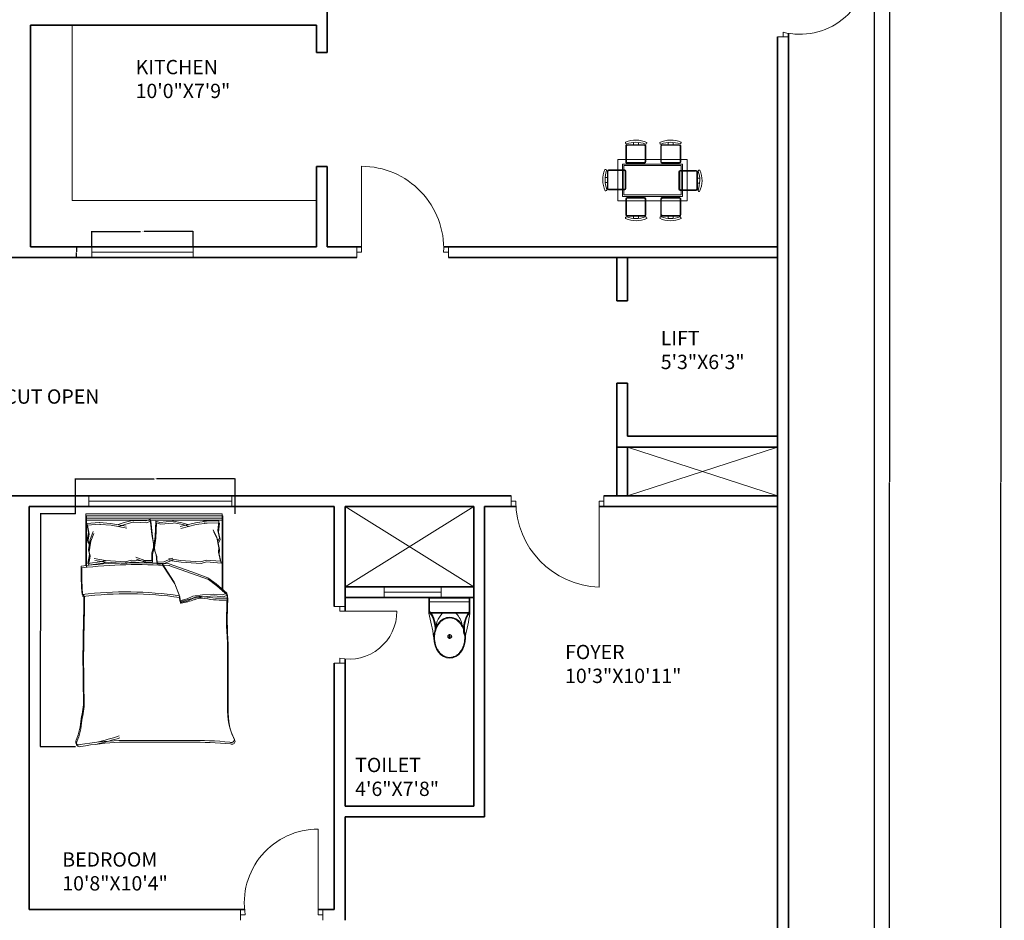
# Model space of a CAD drawing. Units: inches. Extents: x 1520 to 3401, y 1570 to 3432.
# Tile 6 of 15: x 2022 to 2435, y 2061 to 2438. Entities that reach past the tile are written whole.
import ezdxf

# ---------------------------------------------------------------- set-up
doc = ezdxf.new("R2010")
doc.units = ezdxf.units.IN
for name, color, linetype, lineweight in [('A-ANNO-DIMS', 2, 'Continuous', 18), ('A-AREA-IDEN', 7, 'Continuous', 18), ('A-DOOR', 3, 'Continuous', 18), ('A-FLOR-CASE', 8, 'Continuous', 18), ('A-FLOR-EDGE', 7, 'Continuous', 25), ('A-FLOR-EVTR', 7, 'Continuous', 35), ('A-FLOR-FIXT', 9, 'Continuous', 18), ('A-FLOR-OPEN', 8, 'Continuous', 13), ('A-FURN', 8, 'Continuous', 13), ('A-GLAZ', 4, 'Continuous', 18), ('A-WALL', 7, 'Continuous', 35)]:
    doc.layers.add(name, color=color, linetype=linetype, lineweight=lineweight)
doc.styles.get("Standard").update_dxf_attribs({"font": 'arial.ttf'})
doc.dimstyles.get("Standard").update_dxf_attribs({"dimtxt": 0.18, "dimasz": 0.18, "dimexe": 0.18, "dimexo": 0.0625, "dimgap": 0.09, "dimtad": 0, "dimtih": 1, "dimtoh": 1, "dimdec": 4, "dimzin": 0, "dimdsep": 46, "dimtxsty": 'Standard', "dimcen": 0.09, "dimadec": 0, "dimazin": 0, "dimtfac": 1, "dimtdec": 4, "dimtofl": 0, "dimtmove": 0, "dimatfit": 3, "dimfxl": 1, "dimtolj": 1, "dimtzin": 0, "dimarcsym": 0})

# ---------------------------------------------------------------- blocks, each defined once
blk = doc.blocks.new('A$C31115884')
for p, q in [((258, 466), (258, 523)), ((283, 498), (223, 498)), ((0, 200), (0, 0)), ((520, 200), (0, 200)), ((10, 190), (10, 10)), ((510, 190), (10, 190)), ((510, 10), (510, 190)), ((520, 0), (520, 200)), ((510, 54), (0, 54)), ((10, 10), (510, 10)), ((0, 0), (520, 0))]:
    blk.add_line(p, q)
blk.add_circle((256, 496), 23.6)
for centre, radius, start, end in [((2778, -205), 2807, 165.4549, 171.7133), ((3237, 905), 2807, 188.2867, 194.5451), ((-295, 403), 365, 324.2091, 9.3499), ((-295, 403), 375, 324.2091, 9.3499), ((139, 406), 293, 315.8436, 2.6563), ((806, 403), 375, 179.2036, 215.7909), ((806, 403), 365, 170.6501, 215.7909), ((384, 406), 293, 190.2774, 224.1564)]:
    blk.add_arc(centre, radius, start, end)
blk.add_ellipse((256, 510), major_axis=(0, -261), ratio=0.772727)
blk.add_open_spline([(256, 259), (263, 259), (270, 260), (288, 262), (299, 265), (320, 273), (330, 278), (350, 291), (360, 299), (378, 316), (386, 326), (402, 347), (409, 358), (421, 383), (427, 395), (436, 422), (440, 436), (445, 465), (447, 480), (448, 509), (448, 524), (445, 553), (443, 568), (436, 596), (432, 610), (422, 636), (416, 649), (402, 672), (395, 683), (379, 703), (370, 712), (351, 728), (341, 735), (321, 746), (310, 751), (289, 757), (278, 759), (256, 761), (245, 761), (223, 757), (212, 754), (191, 746), (181, 741), (161, 728), (151, 720), (133, 703), (125, 693), (110, 672), (103, 660), (90, 636), (85, 623), (76, 596), (72, 582), (67, 553), (66, 538), (64, 509), (65, 494), (68, 465), (70, 450), (77, 422), (81, 408), (91, 382), (97, 370), (111, 346), (118, 335), (135, 316), (144, 307), (162, 291), (172, 284), (193, 273), (203, 269), (225, 262), (236, 260), (250, 259), (253, 259), (256, 259)], degree=3, knots=[0, 0, 0, 0, 0.110105, 0.110105, 0.285049, 0.285049, 0.459994, 0.459994, 0.634938, 0.634938, 0.809882, 0.809882, 0.984827, 0.984827, 1.159771, 1.159771, 1.334715, 1.334715, 1.50966, 1.50966, 1.684604, 1.684604, 1.859549, 1.859549, 2.034493, 2.034493, 2.209437, 2.209437, 2.384382, 2.384382, 2.559326, 2.559326, 2.73427, 2.73427, 2.909215, 2.909215, 3.084159, 3.084159, 3.259103, 3.259103, 3.434048, 3.434048, 3.608992, 3.608992, 3.783936, 3.783936, 3.958881, 3.958881, 4.133825, 4.133825, 4.30877, 4.30877, 4.483714, 4.483714, 4.658658, 4.658658, 4.833603, 4.833603, 5.008547, 5.008547, 5.183491, 5.183491, 5.358436, 5.358436, 5.53338, 5.53338, 5.708324, 5.708324, 5.883269, 5.883269, 6.058213, 6.058213, 6.233158, 6.233158, 6.283185, 6.283185, 6.283185, 6.283185])
blk = doc.blocks.new('DOOR-SWING-36-16')
for p, q in [((0, 33.75), (0, 38.25)), ((0, 38.25), (0, 36)), ((38.88, 38.25), (38.88, 33.75)), ((0, 36), (2, 36)), ((38.88, 36), (36.88, 36)), ((36.88, 36), (36.88, 0)), ((38.88, 33.75), (38.88, 36)), ((38.88, 36), (38.88, 36))]:
    blk.add_line(p, q)
blk.add_arc((38.02, 36), 36.02, 180, 268.1872)
blk = doc.blocks.new('DOOR-SWING-36-18')
for p, q in [((32.58, 2.25), (32.58, 38.25)), ((0, 4.5), (0, 0)), ((34.58, 4.5), (34.58, 0)), ((0, 0), (0, 2.25)), ((0, 2.25), (2, 2.25)), ((34.58, 2.25), (32.58, 2.25)), ((34.58, 0), (34.58, 2.25))]:
    blk.add_line(p, q)
blk.add_arc((32.58, 7.26), 30.99, 90, 189.3104)
blk = doc.blocks.new('DOOR-SWING-24-19')
for p, q in [((4.5, 23.7), (0, 23.7)), ((0, 23.7), (2.25, 23.7)), ((2.25, 23.7), (2.25, 21.7)), ((2.25, 21.7), (26.25, 21.7)), ((0, 0), (4.5, 0)), ((2.25, 0), (2.25, 2)), ((4.5, 0), (2.25, 0))]:
    blk.add_line(p, q)
blk.add_arc((6.17, 21.7), 20.08, 258.7571, 0)
blk = doc.blocks.new('DOOR-SWING-36-20')
for p, q in [((2, 2.25), (2, 38.25)), ((0, 4.5), (0, 0)), ((38.43, 4.5), (38.43, 0)), ((0, 0), (0, 2.25)), ((0, 2.25), (2, 2.25)), ((38.43, 2.25), (36.43, 2.25)), ((38.43, 0), (38.43, 2.25))]:
    blk.add_line(p, q)
blk.add_arc((2, 3.79), 34.46, 357.4431, 90)
blk = doc.blocks.new('DOOR-SWING-36-23')
for p, q in [((0, 32.12), (4.5, 32.12)), ((4.5, 32.12), (2.25, 32.12)), ((2.25, 32.12), (2.25, 30.12)), ((2.25, 30.12), (38.25, 30.12)), ((4.5, 0), (0, 0)), ((0, 0), (2.25, 0)), ((2.25, 0), (2.25, 2))]:
    blk.add_line(p, q)
blk.add_arc((9.27, 30.12), 28.98, 255.986, 0)
blk = doc.blocks.new('WIN-PLAN-24-01')
for p, q in [((0, 4.5), (0, 0)), ((24, 2.25), (24, 4.5)), ((24, 4.5), (24, 0)), ((0, 0), (0, 2.25)), ((0, 2.25), (24, 2.25))]:
    blk.add_line(p, q)
blk = doc.blocks.new('WIN-PLAN-60-02')
for p, q in [((4.5, 60), (0, 60)), ((0, 60), (2.25, 60)), ((2.25, 60), (2.25, 0)), ((4.5, 0), (0, 0)), ((2.25, 0), (4.5, 0))]:
    blk.add_line(p, q)
blk = doc.blocks.new('WIN-PLAN-42.5-08')
for p, q in [((0, 4.5), (0, 0)), ((42.53, 0), (42.53, 4.5)), ((0, 0), (0, 2.25)), ((0, 2.25), (0, 2.25)), ((0, 2.25), (42.53, 2.25))]:
    blk.add_line(p, q)
blk = doc.blocks.new('BED-DOUBLE')
for p, q in [((4.17, 75.93), (4.17, 97.64)), ((4.17, 97.64), (61.46, 97.64)), ((4.17, 95.8), (61.46, 95.8)), ((4.44, 75.16), (4.44, 96.87)), ((4.44, 96.87), (61.73, 96.87)), ((4.44, 95.03), (61.73, 95.03)), ((29.42, 94.7), (31.15, 95.4)), ((31.15, 95.4), (31.84, 88.98)), ((61.46, 97.64), (61.46, 65.74)), ((61.73, 96.87), (61.73, 64.97)), ((4.67, 93.64), (9.81, 94.03)), ((4.67, 93.66), (5.36, 89.85)), ((4.94, 92.9), (5.64, 89.08)), ((4.95, 92.87), (10.08, 93.27)), ((9.81, 94.03), (9.93, 94.01)), ((9.93, 94.01), (14.52, 93.66)), ((10.08, 93.27), (10.21, 93.24)), ((10.21, 93.24), (14.79, 92.9)), ((14.52, 93.66), (21.1, 92.45)), ((14.79, 92.9), (21.38, 91.68)), ((17.81, 93.14), (20.24, 94.01)), ((18.08, 92.38), (20.51, 93.24)), ((20.24, 94.01), (23.7, 94.88)), ((20.51, 93.24), (23.98, 94.11)), ((23.7, 94.88), (24.09, 94.88)), ((23.98, 94.11), (24.36, 94.11)), ((24.09, 94.88), (29.42, 94.7)), ((24.36, 94.11), (29.69, 93.94)), ((29.69, 93.94), (31.42, 94.63)), ((31.42, 94.63), (32.12, 88.22)), ((33.54, 94.65), (33.25, 88.21)), ((33.81, 93.88), (33.52, 87.44)), ((35.31, 94.07), (33.54, 94.65)), ((35.59, 93.3), (33.81, 93.88)), ((40.62, 94.57), (35.31, 94.07)), ((40.9, 93.81), (35.59, 93.3)), ((41.01, 94.6), (40.62, 94.57)), ((41.28, 93.83), (40.9, 93.81)), ((44.52, 93.95), (41.01, 94.6)), ((44.79, 93.18), (41.28, 93.83)), ((50.25, 93.96), (43.75, 92.34)), ((50.52, 93.19), (44.03, 91.57)), ((47, 93.23), (44.52, 93.95)), ((47.27, 92.47), (44.79, 93.18)), ((54.8, 94.59), (50.25, 93.96)), ((55.08, 93.82), (50.52, 93.19)), ((60.08, 94.57), (53.6, 94.69)), ((53.6, 94.69), (54.8, 94.59)), ((60.35, 93.81), (53.87, 93.92)), ((53.87, 93.92), (55.08, 93.82)), ((59.12, 87.74), (57.7, 90.95)), ((60.08, 94.57), (59.62, 90.72)), ((60.35, 93.81), (59.9, 89.96)), ((5.36, 89.85), (4.84, 86.73)), ((5.64, 89.08), (5.12, 85.96)), ((5.36, 82.57), (6.06, 86.9)), ((6.06, 86.9), (7.27, 90.2)), ((6.33, 86.14), (7.54, 89.43)), ((31.84, 88.98), (32.54, 85.17)), ((32.12, 88.22), (32.81, 84.4)), ((33.25, 88.21), (32.79, 84.36)), ((33.52, 87.44), (33.07, 83.59)), ((59.39, 86.97), (57.97, 90.18)), ((60.08, 83.46), (59.12, 87.74)), ((60.35, 82.69), (59.39, 86.97)), ((59.62, 90.72), (60.34, 87.64)), ((60.34, 87.64), (59.72, 86.39)), ((59.9, 89.96), (60.61, 86.88)), ((60.61, 86.88), (59.99, 85.62)), ((4.84, 86.73), (5.54, 85.52)), ((5.12, 85.96), (5.81, 84.75)), ((5.64, 81.8), (6.33, 86.14)), ((32.54, 83.61), (31.84, 81.36)), ((32.81, 82.84), (32.12, 80.59)), ((32.54, 85.17), (32.54, 83.61)), ((32.79, 84.36), (32.89, 82.8)), ((32.81, 84.4), (32.81, 82.84)), ((32.89, 82.8), (33.72, 80.59)), ((33.07, 83.59), (33.17, 82.03)), ((59.85, 81.53), (60.08, 83.46)), ((60.12, 80.77), (60.35, 82.69)), ((5.02, 76.85), (5.71, 80.66)), ((5.29, 76.08), (5.98, 79.9)), ((5.71, 80.66), (5.36, 82.57)), ((5.98, 79.9), (5.64, 81.8)), ((7.65, 78.9), (12.48, 78.1)), ((28.9, 78.14), (25.13, 79.45)), ((29.17, 77.37), (25.4, 78.68)), ((31.84, 81.36), (31.84, 78.14)), ((32.12, 80.59), (32.12, 77.37)), ((33.17, 82.03), (34, 79.83)), ((33.72, 80.59), (33.93, 77.39)), ((34, 79.83), (34.2, 76.62)), ((36.87, 77.57), (40.55, 79.11)), ((39.04, 78.9), (43.87, 78.1)), ((60.78, 77.77), (59.85, 81.53)), ((61.05, 77), (60.12, 80.77)), ((11.13, 77.72), (5.02, 76.85)), ((11.4, 76.95), (5.29, 76.08)), ((7.92, 78.14), (12.76, 77.34)), ((12.48, 78.1), (11.13, 77.72)), ((12.76, 77.34), (11.4, 76.95)), ((12.48, 78.1), (20.89, 77.59)), ((12.76, 77.34), (21.16, 76.82)), ((20.89, 77.59), (23.24, 78.25)), ((21.16, 76.82), (23.51, 77.49)), ((23.24, 78.25), (29.39, 77.77)), ((23.51, 77.49), (29.67, 77)), ((31.84, 78.14), (28.9, 78.14)), ((32.12, 77.37), (29.17, 77.37)), ((33.93, 77.39), (36.87, 77.57)), ((34.2, 76.62), (37.14, 76.8)), ((36.28, 76.8), (41.3, 69.01)), ((36.55, 76.03), (41.57, 68.25)), ((37.14, 76.8), (40.82, 78.34)), ((48.73, 73.28), (38.73, 76.8)), ((49, 72.52), (39, 76.03)), ((39.31, 78.14), (44.15, 77.34)), ((43.87, 78.1), (52.28, 77.59)), ((44.15, 77.34), (52.55, 76.82)), ((52.28, 77.59), (54.63, 78.25)), ((52.55, 76.82), (54.9, 77.49)), ((54.63, 78.25), (60.78, 77.77)), ((54.9, 77.49), (61.05, 77)), ((55.41, 70.87), (48.73, 73.28)), ((55.69, 70.1), (49, 72.52)), ((58.94, 68.27), (55.41, 70.87)), ((41.3, 69.01), (43.34, 63.63)), ((41.57, 68.25), (43.62, 62.87)), ((59.21, 67.51), (55.69, 70.1)), ((63.38, 64.38), (58.94, 68.27)), ((63.66, 63.61), (59.21, 67.51)), ((43.34, 63.63), (43.71, 61.22)), ((43.62, 62.87), (43.99, 60.45)), ((46.68, 61.96), (49.1, 63.08)), ((46.96, 61.2), (49.37, 62.31)), ((49.1, 63.08), (53.18, 63.63)), ((49.37, 62.31), (53.46, 62.87)), ((53.18, 63.63), (57.82, 64)), ((53.46, 62.87), (58.1, 63.24)), ((57.82, 64), (61.54, 63.63)), ((58.1, 63.24), (61.81, 62.87)), ((61.54, 63.63), (63.38, 64.38)), ((61.81, 62.87), (63.66, 63.61)), ((63.48, 62.28), (63.38, 64.38, 4.64)), ((63.75, 61.52), (63.66, 63.61, 4.64)), ((43.71, 61.22), (46.68, 61.96)), ((43.99, 60.45), (46.96, 61.2)), ((18.06, 2.64), (47.57, 2.64)), ((18.33, 1.87), (47.84, 1.87))]:
    blk.add_line(p, q)
for centre, radius, start, end in [((102.1, 73.55), 99.87, 178.7218, 185.604), ((25.61, -120.62), 197.77, 86.0865, 96.7821), ((102.37, 72.78), 99.87, 178.7218, 185.604), ((25.88, -121.38), 197.77, 86.0865, 96.7821), ((21.29, -89.76), 154.68, 81.7845, 96.9006), ((21.56, -90.53), 154.68, 81.7845, 96.9006), ((-200.58, 60.27), 203.94, 358.4762, 1.0082), ((-200.3, 59.5), 203.94, 358.4762, 1.0082), ((37.35, 95.86), 35.55, 280.6617, 289.8806), ((52.44, 55.6), 7.46, 78.6608, 113.7384), ((52.72, 54.83), 7.46, 78.6608, 113.7384), ((61.53, 105.62), 43.38, 259.8763, 272.5657), ((61.81, 104.85), 43.38, 259.8763, 272.5657), ((218.51, 54.1), 155.25, 176.9791, 183.8365), ((43.92, 61.15), 0.221, 160.2464, 271.1377), ((44.2, 60.38), 0.221, 160.2464, 271.1377), ((37.62, 95.1), 35.55, 280.6617, 289.8806), ((218.79, 53.34), 155.25, 176.9791, 183.8365), ((581.23, 36.96), 578.22, 178.22771, 181.71854), ((581.51, 36.19), 578.22, 178.22771, 181.71854), ((-5405.34, 16.33), 5469.02, 0.00217, 0.28689), ((-5405.07, 15.56), 5469.02, 0.00217, 0.28689), ((-32.25, 20.29), 35.53, 346.0648, 358.9113), ((-31.97, 19.53), 35.53, 346.0648, 358.9113), ((91.3, 15.32), 27.65, 177.4714, 206.4681), ((91.58, 14.55), 27.65, 177.4714, 206.4681), ((-25.97, 13.39), 28.25, 337.9751, 356.652), ((-25.69, 12.62), 28.25, 337.9751, 356.652), ((-20.65, 126.07), 127.63, 283.3832, 287.7053), ((1.3, 2.07), 1.31, 146.1736, 293.4781), ((1.58, 1.3), 1.31, 146.1736, 293.4781), ((25.69, -143.14), 145.97, 92.9958, 99.4091), ((25.96, -143.9), 145.97, 92.9958, 99.4091), ((-20.37, 125.3), 127.63, 283.3832, 287.7053), ((49.34, -156.85), 159.5, 84.4998, 90.6351), ((49.61, -157.62), 159.5, 84.4998, 90.6351), ((65.23, 3.08), 1.32, 242.6588, 356.02), ((65.5, 2.32), 1.32, 242.6588, 356.02)]:
    blk.add_arc(centre, radius, start, end)
blk = doc.blocks.new('KITCHEN-COUNTER-03')
for p, q in [((0, 0), (0, 73.56)), ((102.45, 0), (0, 0))]:
    blk.add_line(p, q)
blk = doc.blocks.new('DINING-CHAIR-01')
for points in [[(0.47, 8.09, -0.175809), (8.38, 8.03, 0.578392), (8.97, 8.69, 0.214524), (0.06, 8.81, 0.552014), (0.47, 8.09, -0.065079)], [(5.46, 7.77), (5.46, 8.7, -0.064759)], [(8.04, 7.77), (0.7, 7.77, 0.414214), (0.19, 7.26), (0.19, 0.51, 0.414214), (0.7, 0), (8.04, 0, 0.414214), (8.55, 0.51), (8.55, 7.26, 0.414214), (8.04, 7.77)]]:
    blk.add_lwpolyline(points, format="xyb")
blk.add_lwpolyline([(3.41, 8.72), (3.41, 7.77)])
blk.add_lwpolyline([(0.71, 7.54), (7.81, 7.54, -0.414214), (8.32, 7.03), (8.32, 0.74, -0.414214), (7.81, 0.23), (0.71, 0.23, -0.512069), (0.42, 0.74), (0.42, 7.03, -0.512069)], format="xyb", close=True)
blk = doc.blocks.new('DINING-CHAIR-06')
for points in [[(8.29, 1.93, 0.414214), (8.81, 2.45), (8.81, 9.19, 0.414214), (8.29, 9.7), (0.96, 9.7, 0.414214), (0.45, 9.19), (0.45, 2.45, 0.414214), (0.96, 1.93), (8.29, 1.93)], [(8.52, 1.62, -0.175809), (0.62, 1.68, 0.578392), (0.02, 1.02, 0.214524), (8.94, 0.9, 0.552014), (8.52, 1.62, -0.065079)], [(3.53, 1.93), (3.53, 1, -0.064759)]]:
    blk.add_lwpolyline(points, format="xyb")
blk.add_lwpolyline([(8.29, 2.16), (1.19, 2.16, -0.414214), (0.68, 2.68), (0.68, 8.96, -0.414214), (1.19, 9.47), (8.29, 9.47, -0.512069), (8.58, 8.96), (8.58, 2.68, -0.512069)], format="xyb", close=True)
blk.add_lwpolyline([(5.59, 0.99), (5.59, 1.93)])
blk = doc.blocks.new('DINING-TABLE')
for points in [[(0, 17.41), (29.01, 17.41), (29.01, 0), (0, 0)], [(1.93, 15.47), (27.08, 15.47), (27.08, 1.93), (1.93, 1.93)], [(2.51, 14.89), (26.5, 14.89), (26.5, 2.51), (2.51, 2.51)]]:
    blk.add_lwpolyline(points, close=True)
blk = doc.blocks.new('*D69')
at = {"layer": 'A-ANNO-DIMS', "color": 0, "lineweight": -2, "transparency": 16777216}
for p, q in [((2044.99, 2231.14), (2030.2, 2231.14)), ((2030.38, 2230.96), (2030.38, 2182.44)), ((2030.38, 2133.55), (2030.38, 2182.07)), ((2044.99, 2133.37), (2030.2, 2133.37))]:
    blk.add_line(p, q, dxfattribs=at)
at = {"layer": 'A-ANNO-DIMS', "color": 0, "transparency": 16777216}
for points in [[(2030.35, 2230.96), (2030.41, 2230.96), (2030.38, 2231.14)], [(2030.35, 2133.55), (2030.41, 2133.55), (2030.38, 2133.37)]]:
    blk.add_solid(points, dxfattribs=at)
at = {"layer": 'Defpoints', "color": 0, "transparency": 16777216}
for p in [(2030.38, 2231.14), (2045.05, 2231.14), (2045.05, 2133.37)]:
    blk.add_point(p, dxfattribs=at)
at = {"layer": 'A-ANNO-DIMS', "color": 0, "transparency": 16777216, "insert": (2030.38, 2182.26), "char_height": 0.18, "attachment_point": 5}
blk.add_mtext('\\A1;BED 98 TYP.', dxfattribs=at)
blk = doc.blocks.new('*D70')
at = {"layer": 'A-ANNO-DIMS', "color": 0, "lineweight": -2, "transparency": 16777216}
for p, q in [((2045.05, 2231.2), (2045.05, 2245.98)), ((2045.23, 2245.8), (2077.98, 2245.8)), ((2111.79, 2245.8), (2079.04, 2245.8)), ((2111.97, 2231.2), (2111.97, 2245.98))]:
    blk.add_line(p, q, dxfattribs=at)
at = {"layer": 'A-ANNO-DIMS', "color": 0, "transparency": 16777216}
for points in [[(2045.23, 2245.83), (2045.23, 2245.77), (2045.05, 2245.8)], [(2111.79, 2245.83), (2111.79, 2245.77), (2111.97, 2245.8)]]:
    blk.add_solid(points, dxfattribs=at)
at = {"layer": 'Defpoints', "color": 0, "transparency": 16777216}
for p in [(2111.97, 2245.8), (2045.05, 2231.14), (2111.97, 2231.14)]:
    blk.add_point(p, dxfattribs=at)
at = {"layer": 'A-ANNO-DIMS', "color": 0, "transparency": 16777216, "insert": (2078.51, 2245.8), "char_height": 0.18, "attachment_point": 5}
blk.add_mtext('\\A1;67 TYP.', dxfattribs=at)
blk = doc.blocks.new('*D147')
at = {"layer": 'A-ANNO-DIMS', "color": 0, "lineweight": -2, "transparency": 16777216}
for p, q in [((2051.85, 2343.24), (2051.85, 2349.74)), ((2052.03, 2349.56), (2072.36, 2349.56)), ((2094.2, 2349.56), (2073.87, 2349.56)), ((2094.38, 2343.24), (2094.38, 2349.74))]:
    blk.add_line(p, q, dxfattribs=at)
at = {"layer": 'A-ANNO-DIMS', "color": 0, "transparency": 16777216}
for points in [[(2052.03, 2349.59), (2052.03, 2349.53), (2051.85, 2349.56)], [(2094.2, 2349.59), (2094.2, 2349.53), (2094.38, 2349.56)]]:
    blk.add_solid(points, dxfattribs=at)
at = {"layer": 'Defpoints', "color": 0, "transparency": 16777216}
for p in [(2094.38, 2349.56), (2051.85, 2343.18), (2094.38, 2343.18)]:
    blk.add_point(p, dxfattribs=at)
at = {"layer": 'A-ANNO-DIMS', "color": 0, "transparency": 16777216, "insert": (2073.12, 2349.56), "char_height": 0.18, "attachment_point": 5}
blk.add_mtext('\\A1;W8 43 TYP.', dxfattribs=at)
blk = doc.blocks.new('*D148')
at = {"layer": 'A-ANNO-DIMS', "color": 0, "lineweight": -2, "transparency": 16777216}
for p, q in [((2051.79, 2343.18), (2045.29, 2343.18)), ((2045.47, 2343), (2045.47, 2341.11)), ((2051.79, 2338.68), (2045.29, 2338.68)), ((2045.47, 2338.86), (2045.47, 2340.75))]:
    blk.add_line(p, q, dxfattribs=at)
at = {"layer": 'A-ANNO-DIMS', "color": 0, "transparency": 16777216}
for points in [[(2045.44, 2343), (2045.5, 2343), (2045.47, 2343.18)], [(2045.44, 2338.86), (2045.5, 2338.86), (2045.47, 2338.68)]]:
    blk.add_solid(points, dxfattribs=at)
at = {"layer": 'Defpoints', "color": 0, "transparency": 16777216}
for p in [(2045.47, 2343.18), (2051.85, 2343.18), (2051.85, 2338.68)]:
    blk.add_point(p, dxfattribs=at)
at = {"layer": 'A-ANNO-DIMS', "color": 0, "transparency": 16777216, "insert": (2045.47, 2340.93), "char_height": 0.18, "attachment_point": 5}
blk.add_mtext('\\A1;5 TYP.', dxfattribs=at)
blk = doc.blocks.new('*D182')
at = {"layer": 'A-ANNO-DIMS', "color": 0, "lineweight": -2, "transparency": 16777216}
for p, q in [((2380.18, 2733.18), (2433.39, 2733.18)), ((2433.21, 2733), (2433.21, 2244.61)), ((2433.21, 1755.86), (2433.21, 2244.25)), ((2344.18, 1755.68), (2433.39, 1755.68))]:
    blk.add_line(p, q, dxfattribs=at)
at = {"layer": 'A-ANNO-DIMS', "color": 0, "transparency": 16777216}
for points in [[(2433.18, 2733), (2433.24, 2733), (2433.21, 2733.18)], [(2433.18, 1755.86), (2433.24, 1755.86), (2433.21, 1755.68)]]:
    blk.add_solid(points, dxfattribs=at)
at = {"layer": 'Defpoints', "color": 0, "transparency": 16777216}
for p in [(2380.11, 2733.18), (2344.11, 1755.68), (2433.21, 1755.68)]:
    blk.add_point(p, dxfattribs=at)
at = {"layer": 'A-ANNO-DIMS', "color": 0, "transparency": 16777216, "insert": (2433.21, 2244.43), "char_height": 0.18, "attachment_point": 5}
blk.add_mtext('\\A1;977.5', dxfattribs=at)
blk = doc.blocks.new('*D192')
at = {"layer": 'A-ANNO-DIMS', "color": 0, "lineweight": -2, "transparency": 16777216}
for p, q in [((2467.84, 2733.18), (2386.32, 2733.18)), ((2386.5, 2733), (2386.5, 2244.61)), ((2386.5, 1755.86), (2386.5, 2244.25)), ((2503.84, 1755.68), (2386.32, 1755.68))]:
    blk.add_line(p, q, dxfattribs=at)
at = {"layer": 'A-ANNO-DIMS', "color": 0, "transparency": 16777216}
for points in [[(2386.47, 2733), (2386.53, 2733), (2386.5, 2733.18)], [(2386.47, 1755.86), (2386.53, 1755.86), (2386.5, 1755.68)]]:
    blk.add_solid(points, dxfattribs=at)
at = {"layer": 'Defpoints', "color": 0, "transparency": 16777216}
for p in [(2467.9, 2733.18), (2386.5, 1755.68), (2503.9, 1755.68)]:
    blk.add_point(p, dxfattribs=at)
at = {"layer": 'A-ANNO-DIMS', "color": 0, "transparency": 16777216, "insert": (2386.5, 2244.43), "char_height": 0.18, "attachment_point": 5}
blk.add_mtext('\\A1;977.5', dxfattribs=at)

msp = doc.modelspace()

# ---------------------------------------------------------------- linework, layer by layer
at = {"layer": 'A-FLOR-EDGE'}
msp.add_line((2380.1128, 2733.1786), (2380.1128, 1791.6786), dxfattribs=at)
at = {"layer": 'A-FLOR-EVTR'}
for p, q in [((2272.1128, 2320.4639), (2272.1128, 2338.6786)), ((2339.6128, 2338.6786), (2276.6128, 2338.6786)), ((2276.6128, 2338.6786), (2276.6128, 2320.4639)), ((2272.1128, 2320.4639), (2276.6128, 2320.4639)), ((2272.1128, 2259.1786), (2272.1128, 2286.025)), ((2276.6128, 2286.025), (2272.1128, 2286.025)), ((2276.6128, 2286.025), (2276.6128, 2263.6786)), ((2276.6128, 2263.6786), (2339.6128, 2263.6786)), ((2276.6128, 2259.1786), (2272.1128, 2259.1786)), ((2272.1128, 2259.1786), (2272.1128, 2238.6786)), ((2339.6128, 2259.1786), (2276.6128, 2259.1786)), ((2276.6128, 2259.1786), (2276.6128, 2238.6786))]:
    msp.add_line(p, q, dxfattribs=at)
at = {"layer": 'A-FLOR-OPEN'}
for p, q in [((2339.6128, 2259.1786), (2276.6128, 2238.6786)), ((2276.6128, 2259.1786), (2339.6128, 2238.6786)), ((2212.1128, 2200.5887), (2158.1128, 2234.1786)), ((2158.1128, 2200.5887), (2212.1128, 2234.1786))]:
    msp.add_line(p, q, dxfattribs=at)
at = {"layer": 'A-FURN'}
for points in [[(2290.7496, 2386.2682, -0.57839206), (2290.151, 2386.9264, -0.21452438), (2299.0703, 2387.0461, -0.55201397), (2298.6513, 2386.328, 0.1758092), (2290.7496, 2386.2682)], [(2298.4205, 2386.0109, -0.41421356), (2298.9337, 2385.4977), (2298.9337, 2378.7527, -0.41421356), (2298.4205, 2378.2395), (2291.0848, 2378.2395, -0.41421356), (2290.5716, 2378.7527), (2290.5716, 2385.4977, -0.41421356), (2291.0848, 2386.0109), (2298.4205, 2386.0109)], [(2293.6615, 2386.0109), (2293.6615, 2386.9386, 0.06475861)], [(2267.929, 2367.2466, -0.57839206), (2267.2708, 2366.648, -0.21452438), (2267.1511, 2375.5674, -0.55201397), (2267.8692, 2375.1483, 0.17580937), (2267.929, 2367.2466)], [(2268.1863, 2374.9175, -0.41421356), (2268.6995, 2375.4307), (2275.4445, 2375.4307, -0.41421356), (2275.9577, 2374.9175), (2275.9577, 2367.5819, -0.41421356), (2275.4445, 2367.0686), (2268.6995, 2367.0686, -0.41421356), (2268.1863, 2367.5819), (2268.1863, 2374.9175)], [(2306.2787, 2374.8971, -0.17580919), (2306.2189, 2366.9954, 0.57839206), (2306.8771, 2366.3968, 0.21452438), (2306.9968, 2375.3161, 0.55201397), (2306.2787, 2374.8971, -0.06507904)], [(2305.9616, 2374.6663, 0.41421356), (2305.4484, 2375.1795), (2298.7034, 2375.1795, 0.41421356), (2298.1901, 2374.6663), (2298.1901, 2367.3306, 0.41421356), (2298.7034, 2366.8174), (2305.4484, 2366.8174, 0.41421356), (2305.9616, 2367.3306), (2305.9616, 2374.6663)], [(2268.1863, 2370.1585), (2267.2586, 2370.1585, 0.06475861)], [(2305.9616, 2369.9073), (2306.8893, 2369.9073, -0.06475861)], [(2283.7622, 2356.0277), (2276.4265, 2356.0277, -0.41421356), (2275.9133, 2356.5409), (2275.9133, 2363.2859, -0.41421356), (2276.4265, 2363.7991), (2283.7622, 2363.7991, -0.41421356), (2284.2754, 2363.2859), (2284.2754, 2356.5409, -0.41421356), (2283.7622, 2356.0277)], [(2284.0974, 2355.7704, -0.57839206), (2284.696, 2355.1122, -0.21452438), (2275.7767, 2354.9925, -0.55201397), (2276.1957, 2355.7105, 0.17580929), (2284.0974, 2355.7704)], [(2281.1855, 2356.0277), (2281.1855, 2355.0999, 0.06475861)]]:
    msp.add_lwpolyline(points, format="xyb", dxfattribs=at)
for points in [[(2298.4174, 2385.7797), (2291.316, 2385.7797, 0.41421356), (2290.8028, 2385.2665), (2290.8028, 2378.9839, 0.41421356), (2291.316, 2378.4707), (2298.4174, 2378.4707, 0.51206948), (2298.7025, 2378.9839), (2298.7025, 2385.2665, 0.51206948)], [(2268.4175, 2374.9144), (2268.4175, 2367.8131, 0.41421356), (2268.9307, 2367.2999), (2275.2133, 2367.2999, 0.41421356), (2275.7265, 2367.8131), (2275.7265, 2374.9144, 0.51206948), (2275.2133, 2375.1995), (2268.9307, 2375.1995, 0.51206948)], [(2305.7304, 2374.6632), (2305.7304, 2367.5618, -0.41421356), (2305.2172, 2367.0486), (2298.9346, 2367.0486, -0.41421356), (2298.4213, 2367.5618), (2298.4213, 2374.6632, -0.51206948), (2298.9346, 2374.9483), (2305.2172, 2374.9483, -0.51206948)], [(2276.4296, 2356.2589), (2283.5309, 2356.2589, 0.41421356), (2284.0442, 2356.7721), (2284.0442, 2363.0547, 0.41421356), (2283.5309, 2363.5679), (2276.4296, 2363.5679, 0.51206948), (2276.1445, 2363.0547), (2276.1445, 2356.7721, 0.51206948)]]:
    msp.add_lwpolyline(points, format="xyb", close=True, dxfattribs=at)
for points in [[(2295.7149, 2386.9555), (2295.7149, 2386.0109)], [(2267.2417, 2372.2119), (2268.1863, 2372.2119)], [(2306.9062, 2371.9606), (2305.9616, 2371.9606)], [(2279.1321, 2355.0831), (2279.1321, 2356.0277)]]:
    msp.add_lwpolyline(points, dxfattribs=at)
at = {"layer": 'A-WALL'}
for p, q in [((2150.6128, 2445.2565), (2150.6128, 2424.6989)), ((2026.1128, 2436.1786), (2146.1128, 2436.1786)), ((2026.1128, 2436.1786), (2026.1128, 2343.1786)), ((2146.1128, 2436.1786), (2146.1128, 2424.6989)), ((2339.6128, 2431.1873), (2339.6128, 1963.6868)), ((2344.1128, 2432.7197), (2344.1128, 1965.1342)), ((2146.1128, 2424.6989), (2150.6128, 2424.6989)), ((2150.6128, 2376.8563), (2146.1128, 2376.8563)), ((2146.1128, 2376.8563), (2146.1128, 2343.1786)), ((2150.6128, 2376.8563), (2150.6128, 2343.1786)), ((2026.1128, 2343.1786), (2146.1128, 2343.1786)), ((2150.6128, 2343.1786), (2165.0531, 2343.1786)), ((2199.5083, 2343.1786), (2339.6128, 2343.1786)), ((2013.7128, 2338.6786), (2163.0531, 2338.6786)), ((2201.4813, 2338.6786), (2339.6128, 2338.6786)), ((2015.4274, 2238.6786), (2227.7862, 2238.6786)), ((2266.6648, 2238.6786), (2339.6128, 2238.6786)), ((2339.6128, 2238.6786), (2339.6128, 2234.1786)), ((2025.6128, 2234.1786), (2025.6128, 2065.1786)), ((2153.6128, 2234.1786), (2025.6128, 2234.1786)), ((2153.6128, 2192.297), (2153.6128, 2234.1786)), ((2158.1128, 2234.1786), (2158.1128, 2190.297)), ((2212.1128, 2234.1786), (2158.1128, 2234.1786)), ((2212.1128, 2108.5887), (2212.1128, 2234.1786)), ((2216.6128, 2234.1786), (2216.6128, 2104.0887)), ((2229.8566, 2234.1786), (2216.6128, 2234.1786)), ((2339.6128, 2234.1786), (2264.6648, 2234.1786)), ((2158.1128, 2196.0887), (2158.1128, 2200.5887)), ((2158.1128, 2200.5887), (2212.1128, 2200.5887)), ((2212.1128, 2196.0887), (2158.1128, 2196.0887)), ((2212.1128, 2108.5887), (2212.1128, 2196.0887)), ((2158.1128, 2170.282), (2158.1128, 2108.5887)), ((2153.6128, 2065.1786), (2153.6128, 2168.5982)), ((2158.1128, 2108.5887), (2212.1128, 2108.5887)), ((2158.1128, 2104.0887), (2216.6128, 2104.0887)), ((2158.1128, 2104.0887), (2158.1128, 2060.6786)), ((2115.9534, 2065.1786), (2025.6128, 2065.1786)), ((2153.6128, 2065.1786), (2146.8169, 2065.1786))]:
    msp.add_line(p, q, dxfattribs=at)

# ---------------------------------------------------------------- block references
at = {"layer": 'A-DOOR'}
for name, p in [('DOOR-SWING-36-23', (2339.613, 2431.187)), ('DOOR-SWING-36-20', (2163.053, 2338.679)), ('DOOR-SWING-36-16', (2227.786, 2200.429)), ('DOOR-SWING-24-19', (2153.613, 2168.598)), ('DOOR-SWING-36-18', (2114.238, 2060.679))]:
    msp.add_blockref(name, p, dxfattribs=at)
at = {"layer": 'A-FLOR-CASE'}
msp.add_blockref('KITCHEN-COUNTER-03', (2043.66, 2362.615), dxfattribs=at)
at = {"layer": 'A-FLOR-FIXT', "xscale": 0.0330640103915726, "yscale": 0.0330640103915726, "zscale": 0.0330640103915726, "rotation": 180}
msp.add_blockref('A$C31115884', (2210.4756, 2196.0887), dxfattribs=at)
at = {"layer": 'A-FURN'}
for name, p in [('DINING-CHAIR-01', (2275.7216, 2378.2393)), ('DINING-TABLE', (2272.6076, 2362.4093)), ('DINING-CHAIR-06', (2290.1266, 2354.0953)), ('BED-DOUBLE', (2045.151, 2133.4991))]:
    msp.add_blockref(name, p, dxfattribs=at)
at = {"layer": 'A-GLAZ'}
msp.add_blockref('WIN-PLAN-42.5-08', (2051.853, 2338.679), dxfattribs=at)
at = {"layer": 'A-GLAZ', "rotation": 270}
msp.add_blockref('WIN-PLAN-60-02', (2050.6259, 2238.6785), dxfattribs=at)
at = {"layer": 'A-GLAZ', "extrusion": (0, 0, -1), "zscale": -1, "rotation": 180}
msp.add_blockref('WIN-PLAN-24-01', (-2174.4767, 2200.5884), dxfattribs=at)

# ---------------------------------------------------------------- texts
at = {"layer": 'A-AREA-IDEN', "char_height": 6, "attachment_point": 1}
for s, width, insert in [('KITCHEN\\P10\'0"X7\'9"', 211.090017, (2070.2518, 2421.5518)), ('LIFT\\P5\'3"X6\'3"', 86.39077, (2290.5793, 2307.872)), ('CUT OPEN', 203.592059, (2015.1778, 2283.3623)), ('FOYER\\P10\'3"X10\'11"', 106.927965, (2250.4256, 2176.2117)), ('TOILET\\P4\'6"X7\'8" ', 82.314077, (2162.369, 2128.8319)), ('BEDROOM\\P10\'8"X10\'4"', 119.738413, (2039.4891, 2089.186))]:
    msp.add_mtext_dynamic_manual_height_columns(s, width=width, gutter_width=12.5, heights=[0], dxfattribs=dict(at, insert=insert))

# ---------------------------------------------------------------- dimensions: what is measured, and where the dimension line sits
at = {"layer": 'A-ANNO-DIMS'}
for base, p1, p2, picture, middle in [((2433.2128, 1755.6786), (2380.1128, 2733.1786), (2344.1128, 1755.6786), '*D182', (2433.2128, 2244.4286)), ((2386.4982, 1755.6786), (2467.8987, 2733.1786), (2503.8987, 1755.6786), '*D192', (2386.4982, 2244.4286))]:
    dim = msp.add_linear_dim(base=base, p1=p1, p2=p2, angle=90, dimstyle='Standard', override={"dimdec": 1, "dimlfac": 1, "dimrnd": 0, "dimzin": 0, "dimdsep": 46, "dimlunit": 2}, dxfattribs=at)
    dim.commit()
    dim.dimension.update_dxf_attribs({"geometry": picture, "text_midpoint": middle})
for base, p1, p2, text, picture, middle in [((2094.3848, 2349.5584), (2051.853, 2343.1786), (2094.3848, 2343.1786), 'W8 <> TYP.', '*D147', (2073.1189, 2349.5584)), ((2111.9734, 2245.8024), (2045.048, 2231.1376), (2111.9734, 2231.1376), '<> TYP.', '*D70', (2078.5107, 2245.8024))]:
    dim = msp.add_linear_dim(base=base, p1=p1, p2=p2, text=text, dimstyle='Standard', override={"dimdec": 0, "dimlfac": 1, "dimrnd": 0, "dimzin": 0, "dimdsep": 46, "dimlunit": 2}, dxfattribs=at)
    dim.commit()
    dim.dimension.update_dxf_attribs({"geometry": picture, "text_midpoint": middle})
for base, p1, p2, text, picture, middle in [((2045.4732527729, 2343.1786294992), (2051.8530212195, 2338.6786294992), (2051.8530212195, 2343.1786294992), '<> TYP.', '*D148', (2045.4732527729, 2340.9286294992)), ((2030.3833, 2231.1376), (2045.048, 2133.3725), (2045.048, 2231.1376), 'BED <> TYP.', '*D69', (2030.3833, 2182.255))]:
    dim = msp.add_linear_dim(base=base, p1=p1, p2=p2, angle=90, text=text, dimstyle='Standard', override={"dimdec": 0, "dimlfac": 1, "dimrnd": 0, "dimzin": 0, "dimdsep": 46, "dimlunit": 2}, dxfattribs=at)
    dim.commit()
    dim.dimension.update_dxf_attribs({"geometry": picture, "text_midpoint": middle})

doc.saveas('drawing.dxf')
